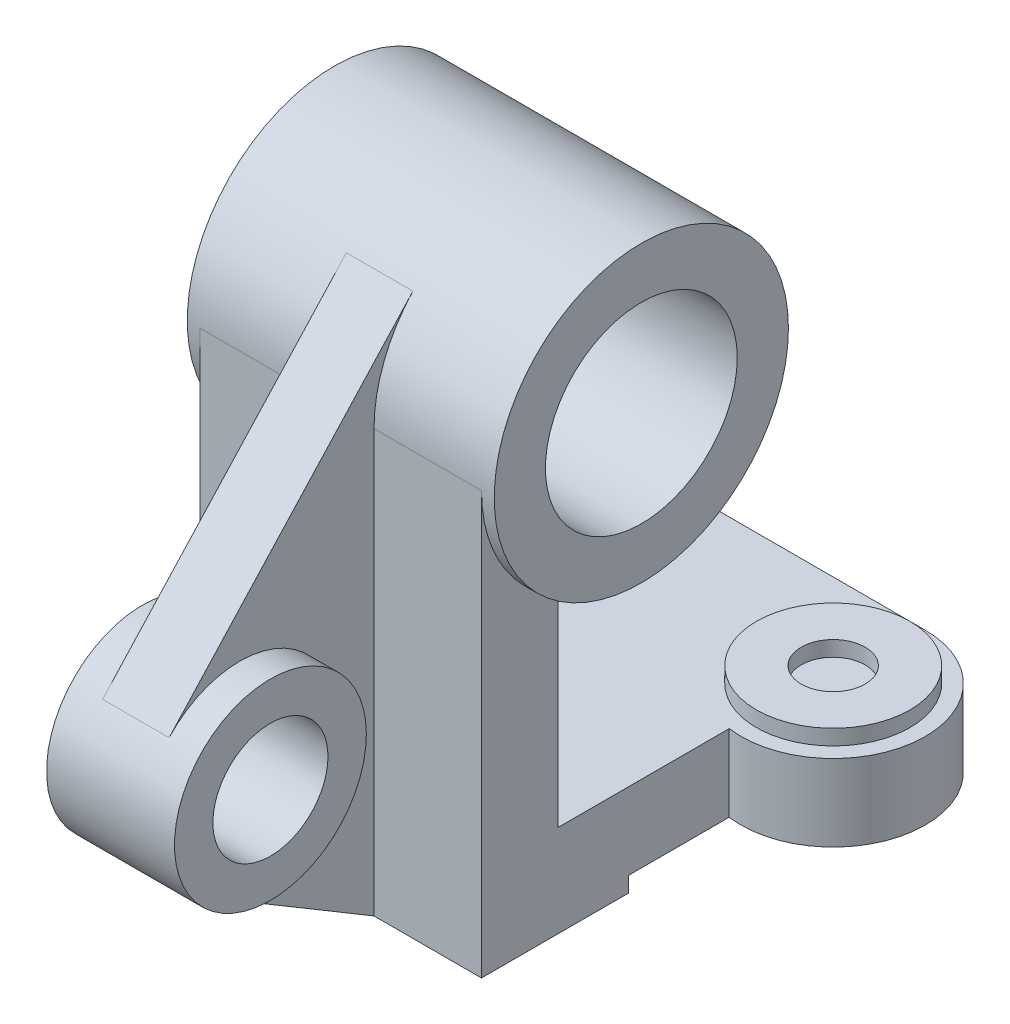
ISO-10303-21;
HEADER;
FILE_DESCRIPTION(('STEP AP214'),'2;1');
FILE_NAME('part.step','',(''),(''),'','','');
FILE_SCHEMA(('AUTOMOTIVE_DESIGN { 1 0 10303 214 1 1 1 1 }'));
ENDSEC;
DATA;
#1=APPLICATION_CONTEXT('core data for automotive mechanical design processes');
#2=APPLICATION_PROTOCOL_DEFINITION('international standard','automotive_design',2000,#1);
#3=PRODUCT_CONTEXT('',#1,'mechanical');
#4=PRODUCT('Part','Part','',(#3));
#5=PRODUCT_RELATED_PRODUCT_CATEGORY('part','',(#4));
#6=PRODUCT_DEFINITION_FORMATION('','',#4);
#7=PRODUCT_DEFINITION_CONTEXT('part definition',#1,'design');
#8=PRODUCT_DEFINITION('design','',#6,#7);
#9=PRODUCT_DEFINITION_SHAPE('','',#8);
#10=(LENGTH_UNIT() NAMED_UNIT(*) SI_UNIT(.MILLI.,.METRE.));
#11=(NAMED_UNIT(*) PLANE_ANGLE_UNIT() SI_UNIT($,.RADIAN.));
#12=(NAMED_UNIT(*) SI_UNIT($,.STERADIAN.) SOLID_ANGLE_UNIT());
#13=UNCERTAINTY_MEASURE_WITH_UNIT(LENGTH_MEASURE(1.E-05),#10,'distance_accuracy_value','');
#14=(GEOMETRIC_REPRESENTATION_CONTEXT(3) GLOBAL_UNCERTAINTY_ASSIGNED_CONTEXT((#13)) GLOBAL_UNIT_ASSIGNED_CONTEXT((#10,
#11,#12)) REPRESENTATION_CONTEXT('',''));
#15=CARTESIAN_POINT('',(0.,0.,0.));
#16=DIRECTION('',(0.,0.,1.));
#17=DIRECTION('',(1.,0.,0.));
#18=AXIS2_PLACEMENT_3D('',#15,#16,#17);
#19=CARTESIAN_POINT('',(55.,0.,57.5));
#20=DIRECTION('',(0.,0.,-1.));
#21=DIRECTION('',(0.,1.,0.));
#22=AXIS2_PLACEMENT_3D('',#19,#20,#21);
#23=PLANE('',#22);
#24=DIRECTION('',(0.,1.,0.));
#25=VECTOR('',#24,1.);
#26=CARTESIAN_POINT('',(-13.,0.,57.5));
#27=LINE('',#26,#25);
#28=CARTESIAN_POINT('',(-13.,-165.,57.5));
#29=VERTEX_POINT('',#28);
#30=CARTESIAN_POINT('',(-13.,0.,57.5));
#31=VERTEX_POINT('',#30);
#32=EDGE_CURVE('E57',#29,#31,#27,.T.);
#33=ORIENTED_EDGE('',*,*,#32,.T.);
#34=DIRECTION('',(-1.,0.,0.));
#35=VECTOR('',#34,1.);
#36=CARTESIAN_POINT('',(55.,0.,57.5));
#37=LINE('',#36,#35);
#38=CARTESIAN_POINT('',(-55.,0.,57.5));
#39=VERTEX_POINT('',#38);
#40=EDGE_CURVE('E205',#31,#39,#37,.T.);
#41=ORIENTED_EDGE('',*,*,#40,.T.);
#42=DIRECTION('',(0.,-1.,0.));
#43=VECTOR('',#42,1.);
#44=CARTESIAN_POINT('',(-55.,0.,57.5));
#45=LINE('',#44,#43);
#46=CARTESIAN_POINT('',(-55.,-165.,57.5));
#47=VERTEX_POINT('',#46);
#48=EDGE_CURVE('E298',#39,#47,#45,.T.);
#49=ORIENTED_EDGE('',*,*,#48,.T.);
#50=DIRECTION('',(-1.,0.,0.));
#51=VECTOR('',#50,1.);
#52=CARTESIAN_POINT('',(55.,-165.,57.5));
#53=LINE('',#52,#51);
#54=EDGE_CURVE('E196',#29,#47,#53,.T.);
#55=ORIENTED_EDGE('',*,*,#54,.F.);
#56=EDGE_LOOP('',(#33,#41,#49,#55));
#57=FACE_BOUND('',#56,.T.);
#58=ADVANCED_FACE('F41',(#57),#23,.F.);
#59=CARTESIAN_POINT('',(60.,0.,0.));
#60=DIRECTION('',(1.,0.,0.));
#61=DIRECTION('',(0.,0.,-1.));
#62=AXIS2_PLACEMENT_3D('',#59,#60,#61);
#63=PLANE('',#62);
#64=CARTESIAN_POINT('',(60.,0.,0.));
#65=DIRECTION('',(1.,0.,0.));
#66=DIRECTION('',(0.,0.,-1.));
#67=AXIS2_PLACEMENT_3D('',#64,#65,#66);
#68=CIRCLE('',#67,57.5);
#69=CARTESIAN_POINT('',(60.,0.,-57.5));
#70=VERTEX_POINT('',#69);
#71=EDGE_CURVE('E211',#70,#70,#68,.T.);
#72=ORIENTED_EDGE('',*,*,#71,.T.);
#73=EDGE_LOOP('',(#72));
#74=FACE_BOUND('',#73,.T.);
#75=CARTESIAN_POINT('',(60.,0.,0.));
#76=DIRECTION('',(1.,0.,0.));
#77=DIRECTION('',(0.,0.,-1.));
#78=AXIS2_PLACEMENT_3D('',#75,#76,#77);
#79=CIRCLE('',#78,37.5);
#80=CARTESIAN_POINT('',(60.,0.,-37.5));
#81=VERTEX_POINT('',#80);
#82=EDGE_CURVE('E202',#81,#81,#79,.T.);
#83=ORIENTED_EDGE('',*,*,#82,.F.);
#84=EDGE_LOOP('',(#83));
#85=FACE_BOUND('',#84,.T.);
#86=ADVANCED_FACE('F246',(#74,#85),#63,.T.);
#87=CARTESIAN_POINT('',(-60.,0.,0.));
#88=DIRECTION('',(1.,0.,0.));
#89=DIRECTION('',(0.,0.,-1.));
#90=AXIS2_PLACEMENT_3D('',#87,#88,#89);
#91=PLANE('',#90);
#92=CARTESIAN_POINT('',(-60.,0.,0.));
#93=DIRECTION('',(1.,0.,0.));
#94=DIRECTION('',(0.,0.,-1.));
#95=AXIS2_PLACEMENT_3D('',#92,#93,#94);
#96=CIRCLE('',#95,57.5);
#97=CARTESIAN_POINT('',(-60.,0.,-57.5));
#98=VERTEX_POINT('',#97);
#99=EDGE_CURVE('E208',#98,#98,#96,.T.);
#100=ORIENTED_EDGE('',*,*,#99,.F.);
#101=EDGE_LOOP('',(#100));
#102=FACE_BOUND('',#101,.T.);
#103=CARTESIAN_POINT('',(-60.,0.,0.));
#104=DIRECTION('',(1.,0.,0.));
#105=DIRECTION('',(0.,0.,-1.));
#106=AXIS2_PLACEMENT_3D('',#103,#104,#105);
#107=CIRCLE('',#106,37.5);
#108=CARTESIAN_POINT('',(-60.,0.,-37.5));
#109=VERTEX_POINT('',#108);
#110=EDGE_CURVE('E204',#109,#109,#107,.T.);
#111=ORIENTED_EDGE('',*,*,#110,.T.);
#112=EDGE_LOOP('',(#111));
#113=FACE_BOUND('',#112,.T.);
#114=ADVANCED_FACE('F255',(#102,#113),#91,.F.);
#115=CARTESIAN_POINT('',(60.,0.,0.));
#116=DIRECTION('',(-1.,0.,0.));
#117=DIRECTION('',(0.,0.,1.));
#118=AXIS2_PLACEMENT_3D('',#115,#116,#117);
#119=CYLINDRICAL_SURFACE('',#118,57.5);
#120=DIRECTION('',(-1.,0.,0.));
#121=VECTOR('',#120,1.);
#122=CARTESIAN_POINT('',(13.,38.9359599221038,42.3112399362668));
#123=LINE('',#122,#121);
#124=CARTESIAN_POINT('',(13.,38.9359599221038,42.3112399362668));
#125=VERTEX_POINT('',#124);
#126=CARTESIAN_POINT('',(-13.,38.9359599221038,42.3112399362668));
#127=VERTEX_POINT('',#126);
#128=EDGE_CURVE('E283',#125,#127,#123,.T.);
#129=ORIENTED_EDGE('',*,*,#128,.F.);
#130=CARTESIAN_POINT('',(13.,0.,0.));
#131=DIRECTION('',(-1.,0.,0.));
#132=DIRECTION('',(0.,0.,-1.));
#133=AXIS2_PLACEMENT_3D('',#130,#131,#132);
#134=CIRCLE('',#133,57.5);
#135=CARTESIAN_POINT('',(13.,0.,57.5));
#136=VERTEX_POINT('',#135);
#137=EDGE_CURVE('E347',#136,#125,#134,.T.);
#138=ORIENTED_EDGE('',*,*,#137,.F.);
#139=CARTESIAN_POINT('',(55.,0.,57.5));
#140=VERTEX_POINT('',#139);
#141=EDGE_CURVE('E64',#140,#136,#37,.T.);
#142=ORIENTED_EDGE('',*,*,#141,.F.);
#143=CARTESIAN_POINT('',(55.,0.,0.));
#144=DIRECTION('',(-1.,0.,0.));
#145=DIRECTION('',(0.,0.,-1.));
#146=AXIS2_PLACEMENT_3D('',#143,#144,#145);
#147=CIRCLE('',#146,57.5);
#148=CARTESIAN_POINT('',(55.,-50.4975246918104,27.5));
#149=VERTEX_POINT('',#148);
#150=EDGE_CURVE('E182',#149,#140,#147,.T.);
#151=ORIENTED_EDGE('',*,*,#150,.F.);
#152=DIRECTION('',(-1.,0.,0.));
#153=VECTOR('',#152,1.);
#154=CARTESIAN_POINT('',(55.,-50.4975246918104,27.5));
#155=LINE('',#154,#153);
#156=CARTESIAN_POINT('',(-55.,-50.4975246918104,27.5));
#157=VERTEX_POINT('',#156);
#158=EDGE_CURVE('E190',#149,#157,#155,.T.);
#159=ORIENTED_EDGE('',*,*,#158,.T.);
#160=CARTESIAN_POINT('',(-55.,0.,0.));
#161=DIRECTION('',(-1.,0.,0.));
#162=DIRECTION('',(0.,0.,-1.));
#163=AXIS2_PLACEMENT_3D('',#160,#161,#162);
#164=CIRCLE('',#163,57.5);
#165=EDGE_CURVE('E293',#157,#39,#164,.T.);
#166=ORIENTED_EDGE('',*,*,#165,.T.);
#167=ORIENTED_EDGE('',*,*,#40,.F.);
#168=CARTESIAN_POINT('',(-13.,0.,0.));
#169=DIRECTION('',(-1.,0.,0.));
#170=DIRECTION('',(0.,0.,-1.));
#171=AXIS2_PLACEMENT_3D('',#168,#169,#170);
#172=CIRCLE('',#171,57.5);
#173=EDGE_CURVE('E336',#31,#127,#172,.T.);
#174=ORIENTED_EDGE('',*,*,#173,.T.);
#175=EDGE_LOOP('',(#129,#138,#142,#151,#159,#166,#167,#174));
#176=FACE_BOUND('',#175,.T.);
#177=ORIENTED_EDGE('',*,*,#71,.F.);
#178=EDGE_LOOP('',(#177));
#179=FACE_BOUND('',#178,.T.);
#180=ORIENTED_EDGE('',*,*,#99,.T.);
#181=EDGE_LOOP('',(#180));
#182=FACE_BOUND('',#181,.T.);
#183=ADVANCED_FACE('F43',(#176,#179,#182),#119,.T.);
#184=CARTESIAN_POINT('',(60.,0.,0.));
#185=DIRECTION('',(-1.,0.,0.));
#186=DIRECTION('',(0.,0.,1.));
#187=AXIS2_PLACEMENT_3D('',#184,#185,#186);
#188=CYLINDRICAL_SURFACE('',#187,37.5);
#189=ORIENTED_EDGE('',*,*,#82,.T.);
#190=EDGE_LOOP('',(#189));
#191=FACE_BOUND('',#190,.T.);
#192=ORIENTED_EDGE('',*,*,#110,.F.);
#193=EDGE_LOOP('',(#192));
#194=FACE_BOUND('',#193,.T.);
#195=ADVANCED_FACE('F261',(#191,#194),#188,.F.);
#196=ORIENTED_EDGE('',*,*,#141,.T.);
#197=DIRECTION('',(0.,1.,0.));
#198=VECTOR('',#197,1.);
#199=CARTESIAN_POINT('',(13.,0.,57.5));
#200=LINE('',#199,#198);
#201=CARTESIAN_POINT('',(13.,-165.,57.5));
#202=VERTEX_POINT('',#201);
#203=EDGE_CURVE('E271',#202,#136,#200,.T.);
#204=ORIENTED_EDGE('',*,*,#203,.F.);
#205=CARTESIAN_POINT('',(55.,-165.,57.5));
#206=VERTEX_POINT('',#205);
#207=EDGE_CURVE('E200',#206,#202,#53,.T.);
#208=ORIENTED_EDGE('',*,*,#207,.F.);
#209=DIRECTION('',(0.,-1.,0.));
#210=VECTOR('',#209,1.);
#211=CARTESIAN_POINT('',(55.,0.,57.5));
#212=LINE('',#211,#210);
#213=EDGE_CURVE('E275',#140,#206,#212,.T.);
#214=ORIENTED_EDGE('',*,*,#213,.F.);
#215=EDGE_LOOP('',(#196,#204,#208,#214));
#216=FACE_BOUND('',#215,.T.);
#217=ADVANCED_FACE('F247',(#216),#23,.F.);
#218=CARTESIAN_POINT('',(55.,-165.,57.5));
#219=DIRECTION('',(0.,1.,0.));
#220=DIRECTION('',(0.,0.,1.));
#221=AXIS2_PLACEMENT_3D('',#218,#219,#220);
#222=PLANE('',#221);
#223=DIRECTION('',(0.,0.,-1.));
#224=VECTOR('',#223,1.);
#225=CARTESIAN_POINT('',(-55.,-165.,57.5));
#226=LINE('',#225,#224);
#227=CARTESIAN_POINT('',(-55.,-165.,0.));
#228=VERTEX_POINT('',#227);
#229=EDGE_CURVE('E301',#47,#228,#226,.T.);
#230=ORIENTED_EDGE('',*,*,#229,.T.);
#231=DIRECTION('',(-1.,0.,0.));
#232=VECTOR('',#231,1.);
#233=CARTESIAN_POINT('',(55.,-165.,0.));
#234=LINE('',#233,#232);
#235=CARTESIAN_POINT('',(55.,-165.,0.));
#236=VERTEX_POINT('',#235);
#237=EDGE_CURVE('E194',#236,#228,#234,.T.);
#238=ORIENTED_EDGE('',*,*,#237,.F.);
#239=DIRECTION('',(0.,0.,-1.));
#240=VECTOR('',#239,1.);
#241=CARTESIAN_POINT('',(55.,-165.,57.5));
#242=LINE('',#241,#240);
#243=EDGE_CURVE('E277',#206,#236,#242,.T.);
#244=ORIENTED_EDGE('',*,*,#243,.F.);
#245=ORIENTED_EDGE('',*,*,#207,.T.);
#246=DIRECTION('',(-1.,0.,0.));
#247=VECTOR('',#246,1.);
#248=CARTESIAN_POINT('',(13.,-165.,57.5));
#249=LINE('',#248,#247);
#250=EDGE_CURVE('E356',#202,#29,#249,.T.);
#251=ORIENTED_EDGE('',*,*,#250,.T.);
#252=ORIENTED_EDGE('',*,*,#54,.T.);
#253=EDGE_LOOP('',(#230,#238,#244,#245,#251,#252));
#254=FACE_BOUND('',#253,.T.);
#255=ADVANCED_FACE('F257',(#254),#222,.F.);
#256=CARTESIAN_POINT('',(55.,-165.,0.));
#257=DIRECTION('',(0.,0.,1.));
#258=DIRECTION('',(1.,0.,0.));
#259=AXIS2_PLACEMENT_3D('',#256,#257,#258);
#260=PLANE('',#259);
#261=DIRECTION('',(0.,1.,0.));
#262=VECTOR('',#261,1.);
#263=CARTESIAN_POINT('',(-55.,-165.,0.));
#264=LINE('',#263,#262);
#265=CARTESIAN_POINT('',(-55.,-159.,0.));
#266=VERTEX_POINT('',#265);
#267=EDGE_CURVE('E181',#228,#266,#264,.T.);
#268=ORIENTED_EDGE('',*,*,#267,.T.);
#269=DIRECTION('',(-1.,0.,0.));
#270=VECTOR('',#269,1.);
#271=CARTESIAN_POINT('',(55.,-159.,0.));
#272=LINE('',#271,#270);
#273=CARTESIAN_POINT('',(55.,-159.,0.));
#274=VERTEX_POINT('',#273);
#275=EDGE_CURVE('E195',#274,#266,#272,.T.);
#276=ORIENTED_EDGE('',*,*,#275,.F.);
#277=DIRECTION('',(0.,1.,0.));
#278=VECTOR('',#277,1.);
#279=CARTESIAN_POINT('',(55.,-165.,0.));
#280=LINE('',#279,#278);
#281=EDGE_CURVE('E290',#236,#274,#280,.T.);
#282=ORIENTED_EDGE('',*,*,#281,.F.);
#283=ORIENTED_EDGE('',*,*,#237,.T.);
#284=EDGE_LOOP('',(#268,#276,#282,#283));
#285=FACE_BOUND('',#284,.T.);
#286=ADVANCED_FACE('F237',(#285),#260,.F.);
#287=CARTESIAN_POINT('',(55.,-159.,0.));
#288=DIRECTION('',(0.,1.,0.));
#289=DIRECTION('',(0.,0.,1.));
#290=AXIS2_PLACEMENT_3D('',#287,#288,#289);
#291=PLANE('',#290);
#292=CARTESIAN_POINT('',(60.,-159.,-75.));
#293=DIRECTION('',(0.,1.,0.));
#294=DIRECTION('',(0.,0.,1.));
#295=AXIS2_PLACEMENT_3D('',#292,#293,#294);
#296=CIRCLE('',#295,36.);
#297=CARTESIAN_POINT('',(60.,-159.,-111.));
#298=VERTEX_POINT('',#297);
#299=CARTESIAN_POINT('',(55.,-159.,-39.3489130600482));
#300=VERTEX_POINT('',#299);
#301=EDGE_CURVE('E309',#298,#300,#296,.F.);
#302=ORIENTED_EDGE('',*,*,#301,.T.);
#303=DIRECTION('',(0.,0.,-1.));
#304=VECTOR('',#303,1.);
#305=CARTESIAN_POINT('',(55.,-159.,0.));
#306=LINE('',#305,#304);
#307=EDGE_CURVE('E287',#274,#300,#306,.T.);
#308=ORIENTED_EDGE('',*,*,#307,.F.);
#309=ORIENTED_EDGE('',*,*,#275,.T.);
#310=DIRECTION('',(0.,0.,-1.));
#311=VECTOR('',#310,1.);
#312=CARTESIAN_POINT('',(-55.,-159.,0.));
#313=LINE('',#312,#311);
#314=CARTESIAN_POINT('',(-55.,-159.,-39.3489130600483));
#315=VERTEX_POINT('',#314);
#316=EDGE_CURVE('E177',#266,#315,#313,.T.);
#317=ORIENTED_EDGE('',*,*,#316,.T.);
#318=CARTESIAN_POINT('',(-60.,-159.,-75.));
#319=DIRECTION('',(0.,1.,0.));
#320=DIRECTION('',(0.,0.,1.));
#321=AXIS2_PLACEMENT_3D('',#318,#319,#320);
#322=CIRCLE('',#321,36.);
#323=CARTESIAN_POINT('',(-60.,-159.,-111.));
#324=VERTEX_POINT('',#323);
#325=EDGE_CURVE('E154',#315,#324,#322,.F.);
#326=ORIENTED_EDGE('',*,*,#325,.T.);
#327=DIRECTION('',(1.,0.,0.));
#328=VECTOR('',#327,1.);
#329=CARTESIAN_POINT('',(-60.,-159.,-111.));
#330=LINE('',#329,#328);
#331=EDGE_CURVE('E676',#324,#298,#330,.T.);
#332=ORIENTED_EDGE('',*,*,#331,.T.);
#333=EDGE_LOOP('',(#302,#308,#309,#317,#326,#332));
#334=FACE_BOUND('',#333,.T.);
#335=ADVANCED_FACE('F225',(#334),#291,.F.);
#336=CARTESIAN_POINT('',(55.,-129.,-75.));
#337=DIRECTION('',(0.,-1.,0.));
#338=DIRECTION('',(0.,0.,-1.));
#339=AXIS2_PLACEMENT_3D('',#336,#337,#338);
#340=PLANE('',#339);
#341=CARTESIAN_POINT('',(60.,-129.,-75.));
#342=DIRECTION('',(0.,-1.,0.));
#343=DIRECTION('',(0.,0.,-1.));
#344=AXIS2_PLACEMENT_3D('',#341,#342,#343);
#345=CIRCLE('',#344,30.);
#346=CARTESIAN_POINT('',(60.,-129.,-105.));
#347=VERTEX_POINT('',#346);
#348=EDGE_CURVE('E11',#347,#347,#345,.F.);
#349=ORIENTED_EDGE('',*,*,#348,.F.);
#350=EDGE_LOOP('',(#349));
#351=FACE_BOUND('',#350,.T.);
#352=CARTESIAN_POINT('',(-60.,-129.,-75.));
#353=DIRECTION('',(0.,-1.,0.));
#354=DIRECTION('',(0.,0.,-1.));
#355=AXIS2_PLACEMENT_3D('',#352,#353,#354);
#356=CIRCLE('',#355,30.);
#357=CARTESIAN_POINT('',(-60.,-129.,-105.));
#358=VERTEX_POINT('',#357);
#359=EDGE_CURVE('E47',#358,#358,#356,.F.);
#360=ORIENTED_EDGE('',*,*,#359,.F.);
#361=EDGE_LOOP('',(#360));
#362=FACE_BOUND('',#361,.T.);
#363=DIRECTION('',(0.,0.,1.));
#364=VECTOR('',#363,1.);
#365=CARTESIAN_POINT('',(55.,-129.,-75.));
#366=LINE('',#365,#364);
#367=CARTESIAN_POINT('',(55.,-129.,-39.3489130600482));
#368=VERTEX_POINT('',#367);
#369=CARTESIAN_POINT('',(55.,-129.,27.5));
#370=VERTEX_POINT('',#369);
#371=EDGE_CURVE('E295',#368,#370,#366,.T.);
#372=ORIENTED_EDGE('',*,*,#371,.F.);
#373=CARTESIAN_POINT('',(60.,-129.,-75.));
#374=DIRECTION('',(0.,1.,0.));
#375=DIRECTION('',(0.,0.,1.));
#376=AXIS2_PLACEMENT_3D('',#373,#374,#375);
#377=CIRCLE('',#376,36.);
#378=CARTESIAN_POINT('',(60.,-129.,-111.));
#379=VERTEX_POINT('',#378);
#380=EDGE_CURVE('E172',#368,#379,#377,.T.);
#381=ORIENTED_EDGE('',*,*,#380,.T.);
#382=DIRECTION('',(-1.,0.,0.));
#383=VECTOR('',#382,1.);
#384=CARTESIAN_POINT('',(-60.,-129.,-111.));
#385=LINE('',#384,#383);
#386=CARTESIAN_POINT('',(-60.,-129.,-111.));
#387=VERTEX_POINT('',#386);
#388=EDGE_CURVE('E161',#379,#387,#385,.T.);
#389=ORIENTED_EDGE('',*,*,#388,.T.);
#390=CARTESIAN_POINT('',(-60.,-129.,-75.));
#391=DIRECTION('',(0.,1.,0.));
#392=DIRECTION('',(0.,0.,1.));
#393=AXIS2_PLACEMENT_3D('',#390,#391,#392);
#394=CIRCLE('',#393,36.);
#395=CARTESIAN_POINT('',(-55.,-129.,-39.3489130600483));
#396=VERTEX_POINT('',#395);
#397=EDGE_CURVE('E153',#387,#396,#394,.T.);
#398=ORIENTED_EDGE('',*,*,#397,.T.);
#399=DIRECTION('',(0.,0.,1.));
#400=VECTOR('',#399,1.);
#401=CARTESIAN_POINT('',(-55.,-129.,-75.));
#402=LINE('',#401,#400);
#403=CARTESIAN_POINT('',(-55.,-129.,27.5));
#404=VERTEX_POINT('',#403);
#405=EDGE_CURVE('E170',#396,#404,#402,.T.);
#406=ORIENTED_EDGE('',*,*,#405,.T.);
#407=DIRECTION('',(-1.,0.,0.));
#408=VECTOR('',#407,1.);
#409=CARTESIAN_POINT('',(55.,-129.,27.5));
#410=LINE('',#409,#408);
#411=EDGE_CURVE('E189',#370,#404,#410,.T.);
#412=ORIENTED_EDGE('',*,*,#411,.F.);
#413=EDGE_LOOP('',(#372,#381,#389,#398,#406,#412));
#414=FACE_BOUND('',#413,.T.);
#415=ADVANCED_FACE('F164',(#351,#362,#414),#340,.F.);
#416=CARTESIAN_POINT('',(55.,-129.,27.5));
#417=DIRECTION('',(0.,0.,1.));
#418=DIRECTION('',(0.,-1.,0.));
#419=AXIS2_PLACEMENT_3D('',#416,#417,#418);
#420=PLANE('',#419);
#421=DIRECTION('',(0.,1.,0.));
#422=VECTOR('',#421,1.);
#423=CARTESIAN_POINT('',(-55.,-129.,27.5));
#424=LINE('',#423,#422);
#425=EDGE_CURVE('E178',#404,#157,#424,.T.);
#426=ORIENTED_EDGE('',*,*,#425,.T.);
#427=ORIENTED_EDGE('',*,*,#158,.F.);
#428=DIRECTION('',(0.,1.,0.));
#429=VECTOR('',#428,1.);
#430=CARTESIAN_POINT('',(55.,-129.,27.5));
#431=LINE('',#430,#429);
#432=EDGE_CURVE('E186',#370,#149,#431,.T.);
#433=ORIENTED_EDGE('',*,*,#432,.F.);
#434=ORIENTED_EDGE('',*,*,#411,.T.);
#435=EDGE_LOOP('',(#426,#427,#433,#434));
#436=FACE_BOUND('',#435,.T.);
#437=ADVANCED_FACE('F222',(#436),#420,.F.);
#438=CARTESIAN_POINT('',(55.,0.,0.));
#439=DIRECTION('',(1.,0.,0.));
#440=DIRECTION('',(0.,0.,-1.));
#441=AXIS2_PLACEMENT_3D('',#438,#439,#440);
#442=PLANE('',#441);
#443=ORIENTED_EDGE('',*,*,#371,.T.);
#444=ORIENTED_EDGE('',*,*,#432,.T.);
#445=ORIENTED_EDGE('',*,*,#150,.T.);
#446=ORIENTED_EDGE('',*,*,#213,.T.);
#447=ORIENTED_EDGE('',*,*,#243,.T.);
#448=ORIENTED_EDGE('',*,*,#281,.T.);
#449=ORIENTED_EDGE('',*,*,#307,.T.);
#450=DIRECTION('',(0.,1.,0.));
#451=VECTOR('',#450,1.);
#452=CARTESIAN_POINT('',(55.,-395.740892116254,-39.3489130600482));
#453=LINE('',#452,#451);
#454=EDGE_CURVE('E159',#300,#368,#453,.T.);
#455=ORIENTED_EDGE('',*,*,#454,.T.);
#456=EDGE_LOOP('',(#443,#444,#445,#446,#447,#448,#449,#455));
#457=FACE_BOUND('',#456,.T.);
#458=ADVANCED_FACE('F235',(#457),#442,.T.);
#459=CARTESIAN_POINT('',(-55.,0.,0.));
#460=DIRECTION('',(1.,0.,0.));
#461=DIRECTION('',(0.,0.,-1.));
#462=AXIS2_PLACEMENT_3D('',#459,#460,#461);
#463=PLANE('',#462);
#464=ORIENTED_EDGE('',*,*,#425,.F.);
#465=ORIENTED_EDGE('',*,*,#405,.F.);
#466=DIRECTION('',(0.,1.,0.));
#467=VECTOR('',#466,1.);
#468=CARTESIAN_POINT('',(-55.,-395.740892116254,-39.3489130600483));
#469=LINE('',#468,#467);
#470=EDGE_CURVE('E149',#315,#396,#469,.T.);
#471=ORIENTED_EDGE('',*,*,#470,.F.);
#472=ORIENTED_EDGE('',*,*,#316,.F.);
#473=ORIENTED_EDGE('',*,*,#267,.F.);
#474=ORIENTED_EDGE('',*,*,#229,.F.);
#475=ORIENTED_EDGE('',*,*,#48,.F.);
#476=ORIENTED_EDGE('',*,*,#165,.F.);
#477=EDGE_LOOP('',(#464,#465,#471,#472,#473,#474,#475,#476));
#478=FACE_BOUND('',#477,.T.);
#479=ADVANCED_FACE('F171',(#478),#463,.F.);
#480=CARTESIAN_POINT('',(13.,-64.6069826594976,137.594286914957));
#481=DIRECTION('',(0.,-0.677147129080065,-0.735847651065508));
#482=DIRECTION('',(0.,0.735847651065508,-0.677147129080065));
#483=AXIS2_PLACEMENT_3D('',#480,#481,#482);
#484=PLANE('',#483);
#485=DIRECTION('',(0.,-0.735847651065508,0.677147129080065));
#486=VECTOR('',#485,1.);
#487=CARTESIAN_POINT('',(-13.,-64.6069826594976,137.594286914957));
#488=LINE('',#487,#486);
#489=CARTESIAN_POINT('',(-13.,-64.6069826594976,137.594286914957));
#490=VERTEX_POINT('',#489);
#491=EDGE_CURVE('E358',#127,#490,#488,.T.);
#492=ORIENTED_EDGE('',*,*,#491,.T.);
#493=DIRECTION('',(-1.,0.,0.));
#494=VECTOR('',#493,1.);
#495=CARTESIAN_POINT('',(13.,-64.6069826594976,137.594286914957));
#496=LINE('',#495,#494);
#497=CARTESIAN_POINT('',(13.,-64.6069826594976,137.594286914957));
#498=VERTEX_POINT('',#497);
#499=EDGE_CURVE('E369',#498,#490,#496,.T.);
#500=ORIENTED_EDGE('',*,*,#499,.F.);
#501=DIRECTION('',(0.,-0.735847651065508,0.677147129080065));
#502=VECTOR('',#501,1.);
#503=CARTESIAN_POINT('',(13.,-64.6069826594976,137.594286914957));
#504=LINE('',#503,#502);
#505=EDGE_CURVE('E349',#125,#498,#504,.T.);
#506=ORIENTED_EDGE('',*,*,#505,.F.);
#507=ORIENTED_EDGE('',*,*,#128,.T.);
#508=EDGE_LOOP('',(#492,#500,#506,#507));
#509=FACE_BOUND('',#508,.T.);
#510=ADVANCED_FACE('F376',(#509),#484,.F.);
#511=CARTESIAN_POINT('',(13.,-165.,57.5));
#512=DIRECTION('',(0.,0.858716114628324,-0.512451592326177));
#513=DIRECTION('',(0.,0.512451592326177,0.858716114628324));
#514=AXIS2_PLACEMENT_3D('',#511,#512,#513);
#515=PLANE('',#514);
#516=DIRECTION('',(0.,-0.512451592326177,-0.858716114628324));
#517=VECTOR('',#516,1.);
#518=CARTESIAN_POINT('',(-13.,-165.,57.5));
#519=LINE('',#518,#517);
#520=CARTESIAN_POINT('',(-13.,-122.201854298562,129.216934712232));
#521=VERTEX_POINT('',#520);
#522=EDGE_CURVE('E361',#521,#29,#519,.T.);
#523=ORIENTED_EDGE('',*,*,#522,.T.);
#524=ORIENTED_EDGE('',*,*,#250,.F.);
#525=DIRECTION('',(0.,-0.512451592326177,-0.858716114628324));
#526=VECTOR('',#525,1.);
#527=CARTESIAN_POINT('',(13.,-165.,57.5));
#528=LINE('',#527,#526);
#529=CARTESIAN_POINT('',(13.,-122.201854298562,129.216934712232));
#530=VERTEX_POINT('',#529);
#531=EDGE_CURVE('E353',#530,#202,#528,.T.);
#532=ORIENTED_EDGE('',*,*,#531,.F.);
#533=DIRECTION('',(-1.,0.,0.));
#534=VECTOR('',#533,1.);
#535=CARTESIAN_POINT('',(13.,-122.201854298562,129.216934712232));
#536=LINE('',#535,#534);
#537=EDGE_CURVE('E370',#530,#521,#536,.T.);
#538=ORIENTED_EDGE('',*,*,#537,.T.);
#539=EDGE_LOOP('',(#523,#524,#532,#538));
#540=FACE_BOUND('',#539,.T.);
#541=ADVANCED_FACE('F383',(#540),#515,.F.);
#542=CARTESIAN_POINT('',(13.,0.,0.));
#543=DIRECTION('',(1.,0.,0.));
#544=DIRECTION('',(0.,0.,-1.));
#545=AXIS2_PLACEMENT_3D('',#542,#543,#544);
#546=PLANE('',#545);
#547=ORIENTED_EDGE('',*,*,#137,.T.);
#548=ORIENTED_EDGE('',*,*,#505,.T.);
#549=CARTESIAN_POINT('',(13.,-90.,110.));
#550=DIRECTION('',(-1.,0.,0.));
#551=DIRECTION('',(0.,0.,-1.));
#552=AXIS2_PLACEMENT_3D('',#549,#550,#551);
#553=CIRCLE('',#552,37.5);
#554=EDGE_CURVE('E352',#498,#530,#553,.T.);
#555=ORIENTED_EDGE('',*,*,#554,.T.);
#556=ORIENTED_EDGE('',*,*,#531,.T.);
#557=ORIENTED_EDGE('',*,*,#203,.T.);
#558=EDGE_LOOP('',(#547,#548,#555,#556,#557));
#559=FACE_BOUND('',#558,.T.);
#560=ADVANCED_FACE('F390',(#559),#546,.T.);
#561=CARTESIAN_POINT('',(-13.,0.,0.));
#562=DIRECTION('',(1.,0.,0.));
#563=DIRECTION('',(0.,0.,-1.));
#564=AXIS2_PLACEMENT_3D('',#561,#562,#563);
#565=PLANE('',#564);
#566=ORIENTED_EDGE('',*,*,#173,.F.);
#567=ORIENTED_EDGE('',*,*,#32,.F.);
#568=ORIENTED_EDGE('',*,*,#522,.F.);
#569=CARTESIAN_POINT('',(-13.,-90.,110.));
#570=DIRECTION('',(-1.,0.,0.));
#571=DIRECTION('',(0.,0.,-1.));
#572=AXIS2_PLACEMENT_3D('',#569,#570,#571);
#573=CIRCLE('',#572,37.5);
#574=EDGE_CURVE('E359',#490,#521,#573,.T.);
#575=ORIENTED_EDGE('',*,*,#574,.F.);
#576=ORIENTED_EDGE('',*,*,#491,.F.);
#577=EDGE_LOOP('',(#566,#567,#568,#575,#576));
#578=FACE_BOUND('',#577,.T.);
#579=ADVANCED_FACE('F378',(#578),#565,.F.);
#580=CARTESIAN_POINT('',(25.,-90.,110.));
#581=DIRECTION('',(-1.,0.,0.));
#582=DIRECTION('',(0.,0.,1.));
#583=AXIS2_PLACEMENT_3D('',#580,#581,#582);
#584=CYLINDRICAL_SURFACE('',#583,22.5);
#585=CARTESIAN_POINT('',(25.,-90.,110.));
#586=DIRECTION('',(1.,0.,0.));
#587=DIRECTION('',(0.,0.,-1.));
#588=AXIS2_PLACEMENT_3D('',#585,#586,#587);
#589=CIRCLE('',#588,22.5);
#590=CARTESIAN_POINT('',(25.,-90.,87.5));
#591=VERTEX_POINT('',#590);
#592=EDGE_CURVE('E334',#591,#591,#589,.T.);
#593=ORIENTED_EDGE('',*,*,#592,.T.);
#594=EDGE_LOOP('',(#593));
#595=FACE_BOUND('',#594,.T.);
#596=CARTESIAN_POINT('',(-25.,-90.,110.));
#597=DIRECTION('',(1.,0.,0.));
#598=DIRECTION('',(0.,0.,-1.));
#599=AXIS2_PLACEMENT_3D('',#596,#597,#598);
#600=CIRCLE('',#599,22.5);
#601=CARTESIAN_POINT('',(-25.,-90.,87.5));
#602=VERTEX_POINT('',#601);
#603=EDGE_CURVE('E341',#602,#602,#600,.T.);
#604=ORIENTED_EDGE('',*,*,#603,.F.);
#605=EDGE_LOOP('',(#604));
#606=FACE_BOUND('',#605,.T.);
#607=ADVANCED_FACE('F394',(#595,#606),#584,.F.);
#608=CARTESIAN_POINT('',(25.,-90.,110.));
#609=DIRECTION('',(-1.,0.,0.));
#610=DIRECTION('',(0.,0.,1.));
#611=AXIS2_PLACEMENT_3D('',#608,#609,#610);
#612=CYLINDRICAL_SURFACE('',#611,37.5);
#613=ORIENTED_EDGE('',*,*,#554,.F.);
#614=ORIENTED_EDGE('',*,*,#499,.T.);
#615=ORIENTED_EDGE('',*,*,#574,.T.);
#616=ORIENTED_EDGE('',*,*,#537,.F.);
#617=EDGE_LOOP('',(#613,#614,#615,#616));
#618=FACE_BOUND('',#617,.T.);
#619=CARTESIAN_POINT('',(25.,-90.,110.));
#620=DIRECTION('',(1.,0.,0.));
#621=DIRECTION('',(0.,0.,-1.));
#622=AXIS2_PLACEMENT_3D('',#619,#620,#621);
#623=CIRCLE('',#622,37.5);
#624=CARTESIAN_POINT('',(25.,-90.,72.5));
#625=VERTEX_POINT('',#624);
#626=EDGE_CURVE('E337',#625,#625,#623,.T.);
#627=ORIENTED_EDGE('',*,*,#626,.F.);
#628=EDGE_LOOP('',(#627));
#629=FACE_BOUND('',#628,.T.);
#630=CARTESIAN_POINT('',(-25.,-90.,110.));
#631=DIRECTION('',(1.,0.,0.));
#632=DIRECTION('',(0.,0.,-1.));
#633=AXIS2_PLACEMENT_3D('',#630,#631,#632);
#634=CIRCLE('',#633,37.5);
#635=CARTESIAN_POINT('',(-25.,-90.,72.5));
#636=VERTEX_POINT('',#635);
#637=EDGE_CURVE('E340',#636,#636,#634,.T.);
#638=ORIENTED_EDGE('',*,*,#637,.T.);
#639=EDGE_LOOP('',(#638));
#640=FACE_BOUND('',#639,.T.);
#641=ADVANCED_FACE('F379',(#618,#629,#640),#612,.T.);
#642=CARTESIAN_POINT('',(25.,0.,0.));
#643=DIRECTION('',(1.,0.,0.));
#644=DIRECTION('',(0.,0.,-1.));
#645=AXIS2_PLACEMENT_3D('',#642,#643,#644);
#646=PLANE('',#645);
#647=ORIENTED_EDGE('',*,*,#592,.F.);
#648=EDGE_LOOP('',(#647));
#649=FACE_BOUND('',#648,.T.);
#650=ORIENTED_EDGE('',*,*,#626,.T.);
#651=EDGE_LOOP('',(#650));
#652=FACE_BOUND('',#651,.T.);
#653=ADVANCED_FACE('F514',(#649,#652),#646,.T.);
#654=CARTESIAN_POINT('',(-25.,0.,0.));
#655=DIRECTION('',(1.,0.,0.));
#656=DIRECTION('',(0.,0.,-1.));
#657=AXIS2_PLACEMENT_3D('',#654,#655,#656);
#658=PLANE('',#657);
#659=ORIENTED_EDGE('',*,*,#603,.T.);
#660=EDGE_LOOP('',(#659));
#661=FACE_BOUND('',#660,.T.);
#662=ORIENTED_EDGE('',*,*,#637,.F.);
#663=EDGE_LOOP('',(#662));
#664=FACE_BOUND('',#663,.T.);
#665=ADVANCED_FACE('F417',(#661,#664),#658,.F.);
#666=CARTESIAN_POINT('',(-60.,-395.740892116254,-75.));
#667=DIRECTION('',(0.,1.,0.));
#668=DIRECTION('',(0.,0.,1.));
#669=AXIS2_PLACEMENT_3D('',#666,#667,#668);
#670=CYLINDRICAL_SURFACE('',#669,36.);
#671=ORIENTED_EDGE('',*,*,#325,.F.);
#672=ORIENTED_EDGE('',*,*,#470,.T.);
#673=ORIENTED_EDGE('',*,*,#397,.F.);
#674=DIRECTION('',(0.,1.,0.));
#675=VECTOR('',#674,1.);
#676=CARTESIAN_POINT('',(-60.,-395.740892116254,-111.));
#677=LINE('',#676,#675);
#678=EDGE_CURVE('E330',#324,#387,#677,.T.);
#679=ORIENTED_EDGE('',*,*,#678,.F.);
#680=EDGE_LOOP('',(#671,#672,#673,#679));
#681=FACE_BOUND('',#680,.T.);
#682=ADVANCED_FACE('F151',(#681),#670,.T.);
#683=CARTESIAN_POINT('',(-60.,-395.740892116254,-111.));
#684=DIRECTION('',(0.,0.,-1.));
#685=DIRECTION('',(-1.,0.,0.));
#686=AXIS2_PLACEMENT_3D('',#683,#684,#685);
#687=PLANE('',#686);
#688=ORIENTED_EDGE('',*,*,#331,.F.);
#689=ORIENTED_EDGE('',*,*,#678,.T.);
#690=ORIENTED_EDGE('',*,*,#388,.F.);
#691=DIRECTION('',(0.,1.,0.));
#692=VECTOR('',#691,1.);
#693=CARTESIAN_POINT('',(60.,-395.740892116254,-111.));
#694=LINE('',#693,#692);
#695=EDGE_CURVE('E326',#298,#379,#694,.T.);
#696=ORIENTED_EDGE('',*,*,#695,.F.);
#697=EDGE_LOOP('',(#688,#689,#690,#696));
#698=FACE_BOUND('',#697,.T.);
#699=ADVANCED_FACE('F324',(#698),#687,.T.);
#700=CARTESIAN_POINT('',(60.,-395.740892116254,-75.));
#701=DIRECTION('',(0.,1.,0.));
#702=DIRECTION('',(0.,0.,1.));
#703=AXIS2_PLACEMENT_3D('',#700,#701,#702);
#704=CYLINDRICAL_SURFACE('',#703,36.);
#705=ORIENTED_EDGE('',*,*,#301,.F.);
#706=ORIENTED_EDGE('',*,*,#695,.T.);
#707=ORIENTED_EDGE('',*,*,#380,.F.);
#708=ORIENTED_EDGE('',*,*,#454,.F.);
#709=EDGE_LOOP('',(#705,#706,#707,#708));
#710=FACE_BOUND('',#709,.T.);
#711=ADVANCED_FACE('F424',(#710),#704,.T.);
#712=CARTESIAN_POINT('',(-60.,-123.,-75.));
#713=DIRECTION('',(0.,1.,0.));
#714=DIRECTION('',(0.,0.,1.));
#715=AXIS2_PLACEMENT_3D('',#712,#713,#714);
#716=PLANE('',#715);
#717=CARTESIAN_POINT('',(-60.,-123.,-75.));
#718=DIRECTION('',(0.,1.,0.));
#719=DIRECTION('',(0.,0.,1.));
#720=AXIS2_PLACEMENT_3D('',#717,#718,#719);
#721=CIRCLE('',#720,30.);
#722=CARTESIAN_POINT('',(-60.,-123.,-45.));
#723=VERTEX_POINT('',#722);
#724=EDGE_CURVE('E675',#723,#723,#721,.T.);
#725=ORIENTED_EDGE('',*,*,#724,.T.);
#726=EDGE_LOOP('',(#725));
#727=FACE_BOUND('',#726,.T.);
#728=CARTESIAN_POINT('',(-60.,-123.,-75.));
#729=DIRECTION('',(0.,1.,0.));
#730=DIRECTION('',(0.,0.,1.));
#731=AXIS2_PLACEMENT_3D('',#728,#729,#730);
#732=CIRCLE('',#731,12.5);
#733=CARTESIAN_POINT('',(-60.,-123.,-62.5));
#734=VERTEX_POINT('',#733);
#735=EDGE_CURVE('E670',#734,#734,#732,.T.);
#736=ORIENTED_EDGE('',*,*,#735,.F.);
#737=EDGE_LOOP('',(#736));
#738=FACE_BOUND('',#737,.T.);
#739=ADVANCED_FACE('F431',(#727,#738),#716,.T.);
#740=CARTESIAN_POINT('',(-60.,-123.,-75.));
#741=DIRECTION('',(0.,-1.,0.));
#742=DIRECTION('',(0.,0.,-1.));
#743=AXIS2_PLACEMENT_3D('',#740,#741,#742);
#744=CYLINDRICAL_SURFACE('',#743,30.);
#745=ORIENTED_EDGE('',*,*,#724,.F.);
#746=EDGE_LOOP('',(#745));
#747=FACE_BOUND('',#746,.T.);
#748=ORIENTED_EDGE('',*,*,#359,.T.);
#749=EDGE_LOOP('',(#748));
#750=FACE_BOUND('',#749,.T.);
#751=ADVANCED_FACE('F217',(#747,#750),#744,.T.);
#752=CARTESIAN_POINT('',(-60.,-123.,-75.));
#753=DIRECTION('',(0.,-1.,0.));
#754=DIRECTION('',(0.,0.,-1.));
#755=AXIS2_PLACEMENT_3D('',#752,#753,#754);
#756=CYLINDRICAL_SURFACE('',#755,12.5);
#757=ORIENTED_EDGE('',*,*,#735,.T.);
#758=EDGE_LOOP('',(#757));
#759=FACE_BOUND('',#758,.T.);
#760=CARTESIAN_POINT('',(-60.,-129.,-75.));
#761=DIRECTION('',(0.,1.,0.));
#762=DIRECTION('',(0.,0.,1.));
#763=AXIS2_PLACEMENT_3D('',#760,#761,#762);
#764=CIRCLE('',#763,12.5);
#765=CARTESIAN_POINT('',(-60.,-129.,-62.5));
#766=VERTEX_POINT('',#765);
#767=EDGE_CURVE('E664',#766,#766,#764,.T.);
#768=ORIENTED_EDGE('',*,*,#767,.F.);
#769=EDGE_LOOP('',(#768));
#770=FACE_BOUND('',#769,.T.);
#771=ADVANCED_FACE('F470',(#759,#770),#756,.F.);
#772=CARTESIAN_POINT('',(60.,-123.,-75.));
#773=DIRECTION('',(0.,1.,0.));
#774=DIRECTION('',(0.,0.,1.));
#775=AXIS2_PLACEMENT_3D('',#772,#773,#774);
#776=PLANE('',#775);
#777=CARTESIAN_POINT('',(60.,-123.,-75.));
#778=DIRECTION('',(0.,1.,0.));
#779=DIRECTION('',(0.,0.,1.));
#780=AXIS2_PLACEMENT_3D('',#777,#778,#779);
#781=CIRCLE('',#780,30.);
#782=CARTESIAN_POINT('',(60.,-123.,-45.));
#783=VERTEX_POINT('',#782);
#784=EDGE_CURVE('E175',#783,#783,#781,.T.);
#785=ORIENTED_EDGE('',*,*,#784,.T.);
#786=EDGE_LOOP('',(#785));
#787=FACE_BOUND('',#786,.T.);
#788=CARTESIAN_POINT('',(60.,-123.,-75.));
#789=DIRECTION('',(0.,1.,0.));
#790=DIRECTION('',(0.,0.,1.));
#791=AXIS2_PLACEMENT_3D('',#788,#789,#790);
#792=CIRCLE('',#791,12.5);
#793=CARTESIAN_POINT('',(60.,-123.,-62.5));
#794=VERTEX_POINT('',#793);
#795=EDGE_CURVE('E658',#794,#794,#792,.T.);
#796=ORIENTED_EDGE('',*,*,#795,.F.);
#797=EDGE_LOOP('',(#796));
#798=FACE_BOUND('',#797,.T.);
#799=ADVANCED_FACE('F480',(#787,#798),#776,.T.);
#800=CARTESIAN_POINT('',(60.,-123.,-75.));
#801=DIRECTION('',(0.,-1.,0.));
#802=DIRECTION('',(0.,0.,-1.));
#803=AXIS2_PLACEMENT_3D('',#800,#801,#802);
#804=CYLINDRICAL_SURFACE('',#803,30.);
#805=ORIENTED_EDGE('',*,*,#784,.F.);
#806=EDGE_LOOP('',(#805));
#807=FACE_BOUND('',#806,.T.);
#808=ORIENTED_EDGE('',*,*,#348,.T.);
#809=EDGE_LOOP('',(#808));
#810=FACE_BOUND('',#809,.T.);
#811=ADVANCED_FACE('F490',(#807,#810),#804,.T.);
#812=CARTESIAN_POINT('',(60.,-123.,-75.));
#813=DIRECTION('',(0.,-1.,0.));
#814=DIRECTION('',(0.,0.,-1.));
#815=AXIS2_PLACEMENT_3D('',#812,#813,#814);
#816=CYLINDRICAL_SURFACE('',#815,12.5);
#817=ORIENTED_EDGE('',*,*,#795,.T.);
#818=EDGE_LOOP('',(#817));
#819=FACE_BOUND('',#818,.T.);
#820=CARTESIAN_POINT('',(60.,-129.,-75.));
#821=DIRECTION('',(0.,1.,0.));
#822=DIRECTION('',(0.,0.,1.));
#823=AXIS2_PLACEMENT_3D('',#820,#821,#822);
#824=CIRCLE('',#823,12.5);
#825=CARTESIAN_POINT('',(60.,-129.,-62.5));
#826=VERTEX_POINT('',#825);
#827=EDGE_CURVE('E665',#826,#826,#824,.T.);
#828=ORIENTED_EDGE('',*,*,#827,.F.);
#829=EDGE_LOOP('',(#828));
#830=FACE_BOUND('',#829,.T.);
#831=ADVANCED_FACE('F243',(#819,#830),#816,.F.);
#832=ORIENTED_EDGE('',*,*,#767,.T.);
#833=EDGE_LOOP('',(#832));
#834=FACE_BOUND('',#833,.T.);
#835=ADVANCED_FACE('F227',(#834),#340,.F.);
#836=ORIENTED_EDGE('',*,*,#827,.T.);
#837=EDGE_LOOP('',(#836));
#838=FACE_BOUND('',#837,.T.);
#839=ADVANCED_FACE('F223',(#838),#340,.F.);
#840=CLOSED_SHELL('',(#58,#86,#114,#183,#195,#217,#255,#286,#335,#415,#437,#458,#479,#510,#541,
#560,#579,#607,#641,#653,#665,#682,#699,#711,#739,#751,#771,#799,#811,#831,#835,#839));
#841=MANIFOLD_SOLID_BREP('B2',#840);
#842=ADVANCED_BREP_SHAPE_REPRESENTATION('',(#18,#841),#14);
#843=SHAPE_DEFINITION_REPRESENTATION(#9,#842);
ENDSEC;
END-ISO-10303-21;
